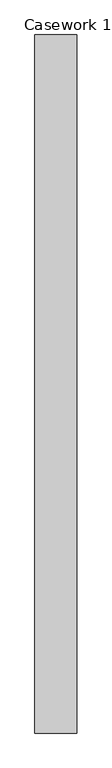
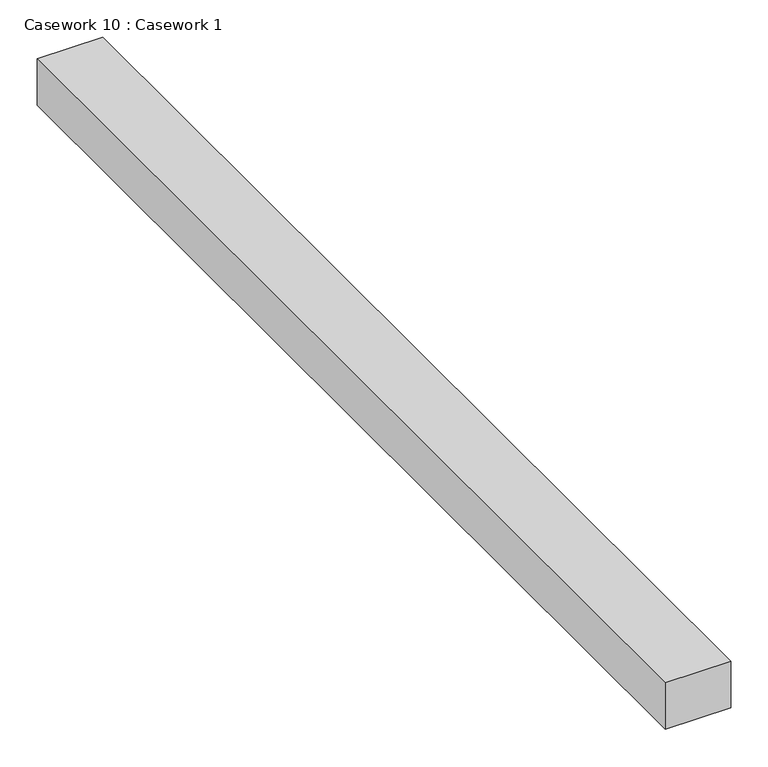
"""IFC4 building model written with IfcOpenShell, lengths in millimetres: furniture geometry, Casework 10 : Casework 1."""

from ifc_helpers import new_model, si_unit, frame, origin, place, context, project, spatial, polyline, outline, extrude, source, transform, mapped, element, save


def casework_10_casework_1_3750556f(model_context):
    return source(origin(), model_context, "Body", "SweptSolid", [
        extrude(outline(polyline([(6919.3559589, 14787.9496924), (6919.3559589, 13098.8496924), (6817.7559589, 13098.8496924), (6817.7559589, 14787.9496924), (6919.3559589, 14787.9496924)])), frame((0.0, 0.0, 3581.4), z_axis=(0.0, 0.0, 1.0), x_axis=(1.0, 0.0, 0.0)), (0.0, 0.0, 1.0), 76.2),
    ])


if __name__ == "__main__":
    model = new_model("IFC4")
    model_context = context("Model", 3, world=origin())
    ifc_project = project(units=[si_unit("LENGTHUNIT", "METRE", prefix="MILLI")], contexts=[model_context])
    site = spatial("IfcSite", under=ifc_project)
    building = spatial("IfcBuilding", under=site)
    placement = place(None, origin())
    casework_10_casework_1_shape = casework_10_casework_1_3750556f(model_context)
    element("IfcFurniture", 1, ObjectType="Casework 10 : Casework 1", at=placement, inside=building, context=model_context, shape_type="MappedRepresentation", body=[
        mapped(casework_10_casework_1_shape, transform((0.0, 0.0, 0.0), x_axis=(1.0, 0.0, 0.0), y_axis=(0.0, 1.0, 0.0), z_axis=(0.0, 0.0, 1.0))),
    ])
    save(model, "model.ifc")

# Revit data of these elements
# Element 1 (IfcFurniture, "Casework 10 : Casework 1")
#   Materials on its faces: "Clad - White"
# Materials
#   "Clad - White": class "Wood", colour RGB 242 242 238, transparency 0, Cost = 0
